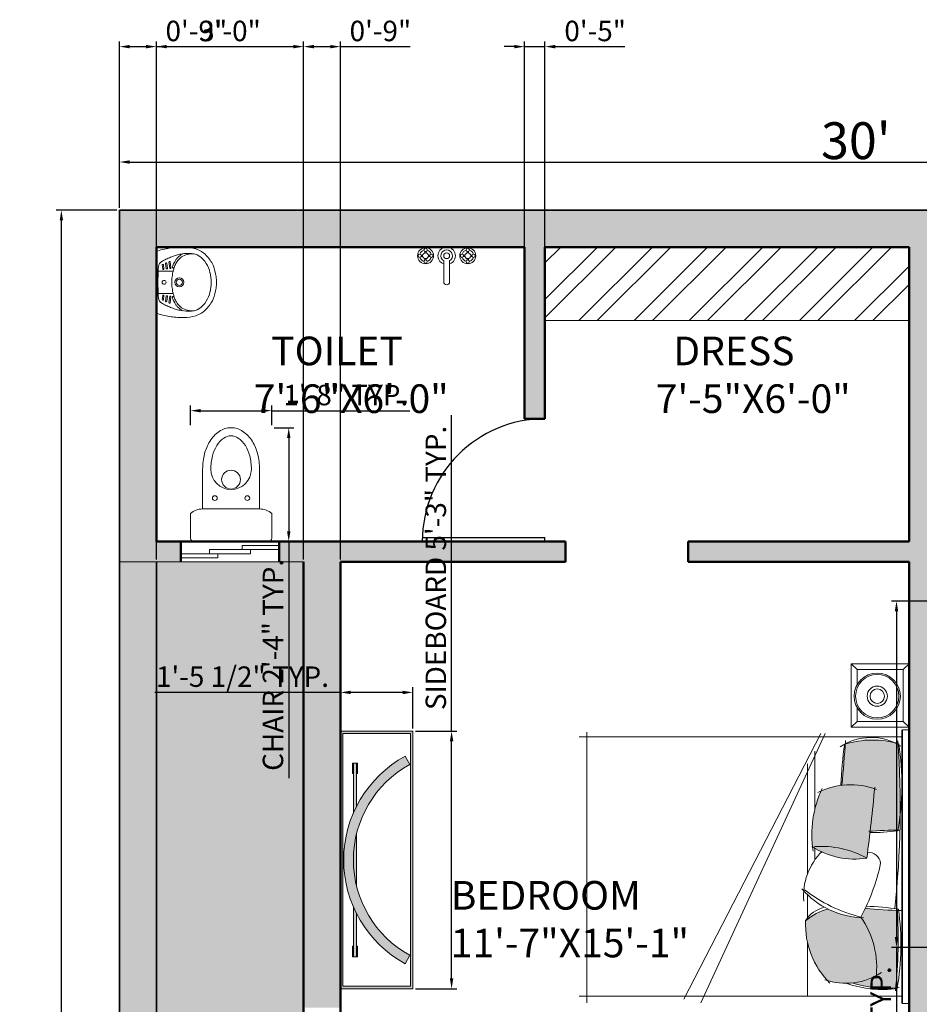
# Model space of a CAD drawing. Units: inches. Extents: x 1734 to 4011, y 1071 to 1891.
# Tile 18 of 27: x 3092 to 3311, y 1638 to 1878. Entities that reach past the tile are written whole.
import ezdxf

# ---------------------------------------------------------------- set-up
doc = ezdxf.new("R2010")
doc.units = ezdxf.units.IN
for name, color, linetype, lineweight in [('0.10', 252, 'Continuous', 9), ('0.15', 34, 'Continuous', 15), ('A-ANNO-DIMS', 2, 'Continuous', 18), ('A-AREA-IDEN', 3, 'Continuous', 18), ('A-DOOR', 3, 'Continuous', 25), ('A-FLOR-FIXT', 9, 'Continuous', 18), ('A-FLOR-PATT', 252, 'Continuous', 13), ('A-FURN', 8, 'Continuous', 18), ('A-FURN-PATT', 252, 'Continuous', 13), ('A-GLAZ', 4, 'Continuous', 18), ('A-WALL', 7, 'Continuous', 50), ('A-WALL-PATT', 8, 'Continuous', 13), ('aparador', 36, 'Continuous', 9), ('C-PROP', 1, 'Continuous', 35), ('moveis', 254, 'Continuous', 5)]:
    doc.layers.add(name, color=color, linetype=linetype, lineweight=lineweight)
doc.styles.get("Standard").update_dxf_attribs({"font": 'arial.ttf'})
doc.dimstyles.new('ISO-25', dxfattribs={"dimtxt": 5, "dimasz": 2.5, "dimexe": 1.25, "dimexo": 0.625, "dimtad": 1, "dimdec": 1, "dimlunit": 3, "dimtxsty": 'Standard', "dimcen": 2.5, "dimclrt": 1, "dimadec": 0, "dimazin": 0, "dimtfac": 1, "dimtdec": 1, "dimtmove": 0, "dimatfit": 3, "dimfxl": 1, "dimarcsym": 0})

# ---------------------------------------------------------------- blocks, each defined once
blk = doc.blocks.new('*D70')
at = {"layer": 'A-ANNO-DIMS', "color": 0, "lineweight": -2, "transparency": 16777216}
for p, q in [((3115.99, 1832.44), (3115.99, 1844.85)), ((3475.99, 1832.44), (3475.99, 1844.85)), ((3118.49, 1843.6), (3473.49, 1843.6))]:
    blk.add_line(p, q, dxfattribs=at)
at = {"layer": 'A-ANNO-DIMS', "color": 0, "transparency": 16777216}
for points in [[(3118.49, 1844.02), (3118.49, 1843.18), (3115.99, 1843.6)], [(3473.49, 1844.02), (3473.49, 1843.18), (3475.99, 1843.6)]]:
    blk.add_solid(points, dxfattribs=at)
at = {"layer": 'Defpoints', "color": 0, "transparency": 16777216}
for p in [(3475.99, 1843.6), (3115.99, 1831.82), (3475.99, 1831.82)]:
    blk.add_point(p, dxfattribs=at)
at = {"layer": 'A-ANNO-DIMS', "color": 0, "transparency": 16777216, "insert": (3295.99, 1848.82), "char_height": 5, "attachment_point": 5}
blk.add_mtext("{\\H1.8x;30'}", dxfattribs=at)
blk = doc.blocks.new('*D66')
at = {"layer": 'A-ANNO-DIMS', "color": 0, "lineweight": -2, "transparency": 16777216}
for p, q in [((3115.37, 1831.82), (3100.52, 1831.82)), ((3101.77, 1114.32), (3101.77, 1829.32)), ((3115.37, 1111.82), (3100.52, 1111.82))]:
    blk.add_line(p, q, dxfattribs=at)
at = {"layer": 'A-ANNO-DIMS', "color": 0, "transparency": 16777216}
for points in [[(3101.36, 1829.32), (3102.19, 1829.32), (3101.77, 1831.82)], [(3101.36, 1114.32), (3102.19, 1114.32), (3101.77, 1111.82)]]:
    blk.add_solid(points, dxfattribs=at)
at = {"layer": 'Defpoints', "color": 0, "transparency": 16777216}
for p in [(3101.77, 1831.82), (3115.99, 1831.82), (3115.99, 1111.82)]:
    blk.add_point(p, dxfattribs=at)
at = {"layer": 'A-ANNO-DIMS', "color": 0, "transparency": 16777216, "insert": (3096.55, 1471.82), "char_height": 5, "attachment_point": 5, "rotation": 90}
blk.add_mtext("{\\H1.8x;60'}", dxfattribs=at)
blk = doc.blocks.new("D2 2'6")
for p, q in [((0, 30), (0, 0)), ((1, 30), (1, 0)), ((0, 0), (1, 0))]:
    blk.add_line(p, q)
blk.add_arc((0, 0), 30, 0, 90)
blk = doc.blocks.new('camita')
at = {"layer": '0.10'}
for p, q in [((-0.85, -0.045), (0.85, -0.045)), ((-0.805, -0.045), (-0.805, -2.0485)), ((0.805, -0.045), (0.805, -2.0485)), ((-0.8271, -0.521), (0.8464, -1.2932)), ((-0.8271, -0.5476), (0.8236, -1.3992)), ((-0.7161, -0.585), (-0.3554, -0.585)), ((-0.1136, -0.585), (-0.0485, -0.585)), ((-0.638, -0.63), (0.0434, -0.63)), ((0.1749, -0.63), (0.3179, -0.63)), ((0.4739, -0.63), (0.805, -0.63)), ((-0.8354, -2), (0.8464, -2))]:
    blk.add_line(p, q, dxfattribs=at)
blk.add_lwpolyline([(-0.85, -0.0405), (0.85, -0.0405), (0.85, 0), (-0.85, 0)], close=True, dxfattribs=at)
for centre, radius, start, end in [((-0.4574, -0.2364), 0.3443, 147.50996, 213.83359), ((-0.3639, -5.8457), 5.7909, 83.80731, 94.12107), ((-0.5104, -1.7232), 1.6781, 80.12554, 98.66187), ((2.3534, -0.0532), 2.5803, 180.10628, 184.38541), ((-1.4396, -0.0609), 1.7117, 352.92911, 0.39592), ((0.4863, -1.6286), 1.5781, 80.16015, 98.05996), ((-0.1997, -0.2266), 0.5864, 163.92635, 197.14087), ((-1.5443, -0.2452), 1.3333, 359.93941, 7.55329), ((1.5815, -0.2893), 1.3353, 170.38021, 178.99138), ((0.4524, -3.0675), 2.9996, 83.90257, 93.67595), ((0.0294, -0.1377), 0.7262, 342.58415, 6.00484), ((0.1326, -0.1696), 0.6307, 339.92303, 8.74334), ((-0.007, -0.258), 0.0828, 100.01798, 179.73597), ((-0.2931, -1.4378), 1.2903, 61.97485, 77.84351), ((0.3203, -0.3944), 0.4043, 341.45245, 33.45121), ((-0.0543, -0.3633), 0.4542, 159.30257, 206.50263), ((-1.3301, -9.6748), 9.4985, 82.27078, 84.93989), ((0.6265, -0.7518), 0.5508, 82.96906, 124.67388), ((0.4585, -0.5454), 0.5842, 151.04555, 184.14969), ((-0.5341, -0.3393), 0.4875, 327.26442, 9.0473), ((-0.1986, -0.2742), 0.5159, 310.73945, 359.05759), ((-0.5673, -0.0868), 0.9057, 321.69527, 346.46261), ((-1.8672, -14.986), 14.6323, 84.65974, 85.75157), ((-0.4598, 1.4861), 1.9092, 260.95299, 268.65169), ((-0.2002, 0.064), 0.6673, 244.78094, 279.06058), ((0.179, -0.272), 0.3828, 224.52836, 275.22287), ((0.4384, -0.4834), 0.1898, 193.68485, 236.70352), ((0.5707, -0.4317), 0.3145, 192.93877, 221.96363), ((0.3612, -0.133), 0.5096, 267.25889, 315.29965)]:
    blk.add_arc(centre, radius, start, end, dxfattribs=at)
blk = doc.blocks.new('VELADOR')
at = {"layer": '0.15'}
for p, q in [((-0.2475, 0), (-0.2025, -0.045)), ((0.2475, 0), (0.2025, -0.045)), ((-0.2025, -0.405), (-0.2475, -0.45)), ((0.2475, -0.45), (0.2025, -0.405))]:
    blk.add_line(p, q, dxfattribs=at)
blk.add_lwpolyline([(-0.2475, 0), (-0.2475, -0.45), (0.2475, -0.45), (0.2475, 0)], close=True, dxfattribs=at)
blk.add_lwpolyline([(0.0921, -0.405), (0.2025, -0.405), (0.2025, -0.045), (-0.2025, -0.045), (-0.2025, -0.405), (-0.0818, -0.405)], dxfattribs=at)
for radius in [0.18, 0.1688, 0.0788, 0.0563]:
    blk.add_circle((0.0052, -0.2474), radius, dxfattribs=at)
blk = doc.blocks.new('Aparador ORGANICA Formatto')
at = {"layer": 'aparador', "ltscale": 0.3}
h = blk.add_hatch(color=256, dxfattribs=at)
h.dxf.hatch_style = 1
h.set_gradient(color1=(118, 213, 123), color2=(52, 168, 57), one_color=1, tint=0.43, name='INVCURVED')
h.paths.add_polyline_path([(0.8, 0.45), (-0.8, 0.45), (-0.8, 0), (0.8, 0)])
h.paths.add_polyline_path([(0.785, 0.435), (0.785, 0.015), (-0.785, 0.015), (-0.785, 0.435)], flags=16)
h.paths.add_polyline_path([(0.2911, 0.3699), (0.5365, 0.3699), (0.5365, 0.3757), (0.6011, 0.3757), (0.6011, 0.3699), (0.6011, 0.3499), (0.6011, 0.3441), (0.5365, 0.3441), (0.5365, 0.3499), (0.3338, 0.3499, -0.150336), (0.6449, 0.0488), (0.5923, 0.0199, 0.208852), (0.1632, 0.3499), (-0.1632, 0.3499, 0.208852), (-0.5923, 0.0199), (-0.6449, 0.0488, -0.150336), (-0.3338, 0.3499), (-0.5365, 0.3499), (-0.5365, 0.3441), (-0.6011, 0.3441), (-0.6011, 0.3499), (-0.6011, 0.3699), (-0.6011, 0.3757), (-0.5365, 0.3757), (-0.5365, 0.3699), (-0.2911, 0.3699, -0.206106)], flags=0)
h = blk.add_hatch(color=256, dxfattribs=at)
h.dxf.hatch_style = 1
h.set_gradient(color1=(135, 92, 69), color2=(0, 0, 0), one_color=1, name='INVCURVED')
h.paths.add_polyline_path([(-0.6449, 0.0488), (-0.5923, 0.0199, -0.590888), (0.5923, 0.0199), (0.6449, 0.0488, 0.590888)])
h = blk.add_hatch(color=256, dxfattribs=at)
h.dxf.hatch_style = 1
h.set_gradient(color1=(178, 189, 189), one_color=1, tint=1, name='CYLINDER')
h.paths.add_polyline_path([(-0.5365, 0.3757), (-0.6011, 0.3757), (-0.6011, 0.3699), (-0.5365, 0.3699)])
h.paths.add_polyline_path([(-0.5365, 0.3499), (-0.6011, 0.3499), (-0.6011, 0.3441), (-0.5365, 0.3441)])
h = blk.add_hatch(color=256, dxfattribs=at)
h.dxf.hatch_style = 1
h.set_gradient(color1=(118, 213, 123), color2=(31, 101, 35), one_color=1, tint=0.26, name='INVCURVED')
h.paths.add_polyline_path([(-0.2911, 0.3699), (-0.6011, 0.3699), (-0.6011, 0.3499), (-0.3338, 0.3499, -0.015999)])
h = blk.add_hatch(color=256, dxfattribs=at)
h.dxf.hatch_style = 1
h.set_gradient(color1=(118, 213, 123), color2=(31, 101, 35), one_color=1, tint=0.26, name='INVCURVED')
h.paths.add_polyline_path([(-0.1632, 0.3499), (0.1632, 0.3499, 0.122516)])
h = blk.add_hatch(color=256, dxfattribs=at)
h.dxf.hatch_style = 1
h.set_gradient(color1=(118, 213, 123), color2=(31, 101, 35), one_color=1, tint=0.26, name='INVCURVED')
h.paths.add_polyline_path([(0.6011, 0.3699), (0.2911, 0.3699, -0.015999), (0.3338, 0.3499), (0.6011, 0.3499)])
h = blk.add_hatch(color=256, dxfattribs=at)
h.dxf.hatch_style = 1
h.set_gradient(color1=(178, 189, 189), one_color=1, tint=1, name='CYLINDER')
h.paths.add_polyline_path([(0.6011, 0.3757), (0.5365, 0.3757), (0.5365, 0.3699), (0.6011, 0.3699)])
h.paths.add_polyline_path([(0.6011, 0.3499), (0.5365, 0.3499), (0.5365, 0.3441), (0.6011, 0.3441)])
for p, q in [((-0.5923, 0.0199), (-0.6449, 0.0488)), ((0.5923, 0.0199), (0.6449, 0.0488))]:
    blk.add_line(p, q, dxfattribs=at)
for points in [[(-0.6011, 0.3699), (-0.6011, 0.3757), (-0.5365, 0.3757), (-0.5365, 0.3699)], [(0.6011, 0.3699), (0.6011, 0.3757), (0.5365, 0.3757), (0.5365, 0.3699)], [(-0.5365, 0.3499), (-0.5365, 0.3441), (-0.6011, 0.3441), (-0.6011, 0.3499)], [(0.5365, 0.3499), (0.5365, 0.3441), (0.6011, 0.3441), (0.6011, 0.3499)]]:
    blk.add_lwpolyline(points, dxfattribs=at)
for radius in [0.7362, 0.6762]:
    blk.add_arc((0, -0.3063), radius, 28.84335, 151.15665, dxfattribs=at)
at = {"layer": 'moveis', "ltscale": 0.3}
for p, q in [((-0.6011, 0.3699), (-0.6011, 0.3499)), ((-0.2911, 0.3699), (-0.6011, 0.3699)), ((0.2911, 0.3699), (0.6011, 0.3699)), ((0.6011, 0.3699), (0.6011, 0.3499)), ((-0.6011, 0.3499), (-0.3338, 0.3499)), ((-0.1632, 0.3499), (0.1632, 0.3499)), ((0.6011, 0.3499), (0.3338, 0.3499))]:
    blk.add_line(p, q, dxfattribs=at)
for points in [[(-0.8, 0), (0.8, 0), (0.8, 0.45), (-0.8, 0.45)], [(-0.785, 0.015), (0.785, 0.015), (0.785, 0.435), (-0.785, 0.435)]]:
    blk.add_lwpolyline(points, close=True, dxfattribs=at)
blk = doc.blocks.new('Faucet - Bathroom top')
for p, q in [((-4.107, 0.125), (-4.375, 0.125)), ((-3.75, 0.4788), (-3.75, 0.75)), ((-3.5, 0.482), (-3.5, 0.75)), ((-3.1461, 0.125), (-2.875, 0.125)), ((3.143, 0.125), (2.875, 0.125)), ((3.5, 0.4788), (3.5, 0.75)), ((3.75, 0.482), (3.75, 0.75)), ((4.1039, 0.125), (4.375, 0.125)), ((-4.1039, -0.125), (-4.375, -0.125)), ((-3.75, -0.4821), (-3.75, -0.75)), ((-3.5, -0.4789), (-3.5, -0.75)), ((-3.143, -0.125), (-2.875, -0.125)), ((-0.5, -0.8639), (-0.5, -4.5)), ((0.5, -4.5), (0.5, -0.8631)), ((3.1461, -0.125), (2.875, -0.125)), ((3.5, -0.4821), (3.5, -0.75)), ((3.75, -0.4789), (3.75, -0.75)), ((4.107, -0.125), (4.375, -0.125))]:
    blk.add_line(p, q)
for centre, radius in [((-3.625, 0), 1.375), ((-4.625, 0), 0.2795), ((-3.625, 0), 0.5), ((-3.625, 1), 0.2795), ((-2.625, 0), 0.2795), ((0, 0), 0.5), ((3.625, 0), 1.375), ((2.625, 0), 0.2795), ((3.625, 0), 0.5), ((3.625, 1), 0.2795), ((4.625, 0), 0.2795), ((-3.625, -1), 0.2795), ((3.625, -1), 0.2795)]:
    blk.add_circle(centre, radius)
for centre, radius, start, end in [((-3.625, 0), 1, 105.2407, 164.2093), ((-3.625, 0), 1, 16.44125, 74.07887), ((0, 0), 1.5, 289.6514, 250.3603), ((0, 0), 1, 300.3431, 239.7554), ((3.625, 0), 1, 106.12, 164.0884), ((3.625, 0), 1, 16.23422, 73.90469), ((-3.625, 0), 1, 196.2342, 253.9047), ((-3.625, 0), 1, 286.12, 344.0884), ((3.625, 0), 1, 196.4413, 254.0789), ((3.625, 0), 1, 285.2407, 344.2093), ((0, -4.5), 0.5, 180, 0)]:
    blk.add_arc(centre, radius, start, end)
blk = doc.blocks.new('lavamanos 2')
at = {"layer": '0.15'}
for p, q in [((0, 0.2335), (0, -0.2335)), ((-0.1127, 0.112), (-0.1067, 0.1581)), ((-0.1037, 0.1109), (-0.0978, 0.157)), ((-0.1304, 0.11), (-0.1315, 0.11)), ((-0.0142, 0.087), (-0.13, 0.086)), ((-0.0857, 0.1085), (-0.0807, 0.1466)), ((-0.0767, 0.1074), (-0.0718, 0.1455)), ((-0.0587, 0.105), (-0.0548, 0.1351)), ((-0.0497, 0.1039), (-0.0458, 0.134)), ((-0.1304, -0.11), (-0.1315, -0.11)), ((-0.0142, -0.087), (-0.13, -0.086)), ((-0.1127, -0.112), (-0.1067, -0.1581)), ((-0.1037, -0.1109), (-0.0978, -0.157)), ((-0.0857, -0.1085), (-0.0807, -0.1466)), ((-0.0767, -0.1074), (-0.0718, -0.1455)), ((-0.0587, -0.105), (-0.0548, -0.1351)), ((-0.0497, -0.1039), (-0.0458, -0.134))]:
    blk.add_line(p, q, dxfattribs=at)
for centre, radius in [((-0.178, 0), 0.035), ((-0.178, 0), 0.0235), ((-0.06, 0), 0.015)]:
    blk.add_circle(centre, radius, dxfattribs=at)
for centre, radius, start, end in [((-0.2419, 0.0663), 0.2023, 108.1945, 135.36859), ((-0.2035, -0.0862), 0.3593, 91.20299, 106.42552), ((-0.2208, -0.6855), 0.9585, 86.55138, 89.41308), ((-0.2121, -0.5476), 0.8204, 83.12241, 86.5796), ((5.8279, 30.215), 30.5319, 258.77821, 258.87599), ((-0.1265, -0.0657), 0.3287, 69.06009, 78.82181), ((-0.0202, 0.212), 0.0314, 54.79491, 69.06009), ((-0.005, 0.2335), 0.005, 0, 54.79491), ((-0.1663, 0.0005), 0.3024, 136.57187, 154.32772), ((-0.2422, 0.0655), 0.1638, 121.99295, 150.58892), ((-0.2657, 0.1037), 0.119, 92.47742, 122.14108), ((-0.2765, 0.0677), 0.1528, 57.2491, 95.54005), ((-0.2442, -0.0128), 0.2368, 77.24819, 96.46321), ((-0.2765, 0.0677), 0.1678, 56.87663, 64.99714), ((-0.3662, -0.002), 0.2627, 40.35252, 49.00458), ((-0.2222, 0.0026), 0.2177, 71.98488, 82.01242), ((-0.3662, -0.002), 0.2777, 40.35252, 49.22548), ((-0.2374, 0.11), 0.0921, 27.31862, 39.11562), ((-0.3103, -0.315), 0.5472, 69.51913, 73.49118), ((-0.2374, 0.11), 0.1071, 27.57433, 39.11562), ((-0.3494, 0.0363), 0.2408, 22.19214, 30.78376), ((-0.2991, -0.2855), 0.5156, 65.23004, 69.53785), ((-0.1022, 0.1575), 0.0045, 352.61396, 172.61396), ((-0.2784, -0.2408), 0.4663, 60.24131, 65.2382), ((-0.0648, 0.1184), 0.049, 1.58272, 68.62081), ((-0.0557, -0.0178), 0.4111, 158.70106, 171.31016), ((-0.1999, 0.0263), 0.2202, 147.11565, 167.44248), ((-0.3494, 0.0363), 0.2258, 22.33605, 30.8927), ((-1.2664, -0.2389), 1.1824, 16.36313, 17.77674), ((-0.1315, 0.117), 0.007, 197.40991, 270.49494), ((0.1853, 0.1648), 0.325, 192.53887, 196.70718), ((-0.1305, 0.117), 0.007, 270.49494, 17.39527), ((-1.2664, -0.2389), 1.1974, 17.39527, 17.80495), ((-0.1082, 0.1115), 0.0045, 172.61396, 352.61396), ((-0.0812, 0.108), 0.0045, 172.61396, 352.61396), ((-0.0763, 0.146), 0.0045, 352.61396, 172.61396), ((-0.0542, 0.1045), 0.0045, 172.61396, 352.61396), ((-0.0503, 0.1345), 0.0045, 352.61396, 172.61396), ((-2.1477, 0.0009), 2.1352, 359.97535, 3.19009), ((-0.2093, 0.0056), 0.2558, 171.31016, 181.26266), ((-0.2093, -0.0056), 0.2558, 178.73734, 188.68984), ((0.4664, -0.0834), 0.8953, 169.86317, 174.65802), ((0.4664, 0.0834), 0.8953, 185.34198, 190.13683), ((0.3887, 0.121), 0.517, 185.50529, 189.81306), ((-0.7181, -0.0071), 0.5987, 0.67647, 3.82165), ((-0.7181, 0.0071), 0.5987, 356.17835, 359.32353), ((-2.1477, -0.0009), 2.1352, 356.80991, 0.02465), ((-0.0557, 0.0178), 0.4111, 188.68984, 201.29894), ((-0.1999, -0.0263), 0.2202, 192.55752, 212.88435), ((0.1853, -0.1648), 0.325, 163.29282, 167.46113), ((0.3887, -0.1209), 0.517, 170.18694, 174.49471), ((-0.1663, -0.0005), 0.3024, 205.67228, 223.42813), ((-0.2422, -0.0655), 0.1638, 209.41108, 238.00705), ((-0.2374, -0.1099), 0.0921, 320.88438, 332.68138), ((-0.3494, -0.0363), 0.2258, 329.1073, 337.66395), ((-0.3494, -0.0363), 0.2408, 329.21624, 337.80786), ((-1.2664, 0.2389), 1.1824, 342.22326, 343.63687), ((-0.1315, -0.117), 0.007, 89.50506, 162.59009), ((-0.1305, -0.117), 0.007, 342.60473, 89.50506), ((-1.2664, 0.2389), 1.1974, 342.19505, 342.60473), ((-0.1082, -0.1115), 0.0045, 7.38604, 187.38604), ((-0.0812, -0.108), 0.0045, 7.38604, 187.38604), ((-0.0763, -0.146), 0.0045, 187.38604, 7.38604), ((-0.0542, -0.1045), 0.0045, 7.38604, 187.38604), ((-0.0503, -0.1345), 0.0045, 187.38604, 7.38604), ((-0.0648, -0.1184), 0.049, 291.37919, 358.41728), ((-0.2419, -0.0663), 0.2023, 224.63141, 251.8055), ((-0.2657, -0.1036), 0.119, 237.85892, 267.52258), ((-0.2765, -0.0677), 0.1528, 264.45995, 302.7509), ((-0.2442, 0.0128), 0.2368, 263.53679, 282.75181), ((-0.2765, -0.0677), 0.1678, 295.00286, 303.12337), ((-0.3662, 0.002), 0.2627, 310.99542, 319.64748), ((-0.2222, -0.0026), 0.2177, 277.98758, 288.01512), ((-0.3662, 0.002), 0.2777, 310.77452, 319.64748), ((-0.3103, 0.315), 0.5472, 286.50882, 290.48087), ((-0.2374, -0.1099), 0.1071, 320.88438, 332.42567), ((-0.2991, 0.2855), 0.5156, 290.46215, 294.76996), ((-0.1022, -0.1575), 0.0045, 187.38604, 7.38604), ((-0.2784, 0.2408), 0.4663, 294.7618, 299.75869), ((-0.2035, 0.0862), 0.3593, 253.57448, 268.79701), ((-0.2208, 0.6855), 0.9585, 270.58692, 273.44862), ((-0.2121, 0.5476), 0.8204, 273.4204, 276.87759), ((5.8279, -30.215), 30.5319, 101.12401, 101.22179), ((-0.1265, 0.0657), 0.3287, 281.17819, 290.93991), ((-0.0202, -0.212), 0.0314, 290.93991, 305.20509), ((-0.005, -0.2335), 0.005, 305.20509, 0)]:
    blk.add_arc(centre, radius, start, end, dxfattribs=at)
blk = doc.blocks.new('rreerr')
blk.add_lwpolyline([(2512.8529, 833.5601, 0.205217), (2512.9279, 833.5883), (2512.9279, 833.7401, 0.414214), (2512.9079, 833.7601), (2512.4479, 833.7601, 0.414214), (2512.4279, 833.7401), (2512.4279, 833.5883, 0.205217), (2512.5029, 833.5601)], format="xyb")
for points in [[(2512.5468, 833.1438, 0.107027), (2512.6056, 833.0819, 0.150548), (2512.6779, 833.0596, 0.150548), (2512.7502, 833.0819, 0.107027), (2512.809, 833.1438, 0.075071), (2512.8412, 833.2206, 0.0618), (2512.8529, 833.3151), (2512.8529, 833.5601), (2512.5029, 833.5601), (2512.5029, 833.3151, 0.0618), (2512.5146, 833.2206, 0.075071)], [(2512.5631, 833.2328, 0.075071), (2512.5895, 833.1698, 0.107027), (2512.6338, 833.1232, 0.150548), (2512.6779, 833.1096, 0.150548), (2512.722, 833.1232, 0.107027), (2512.7663, 833.1698, 0.075071), (2512.7927, 833.2328, 0.0618), (2512.8029, 833.3151, 1), (2512.5529, 833.3151, 0.0618)]]:
    blk.add_lwpolyline(points, format="xyb", close=True)
for centre, radius in [((2512.5779, 833.493), 0.0146), ((2512.7779, 833.493), 0.0146), ((2512.6775, 833.3793), 0.0579)]:
    blk.add_circle(centre, radius)
blk = doc.blocks.new('*D83')
at = {"layer": 'A-ANNO-DIMS', "color": 0, "lineweight": -2, "transparency": 16777216}
for p, q in [((3197.16, 1704.46), (3197.16, 1781.74)), ((3188.34, 1704.46), (3198.41, 1704.46)), ((3197.16, 1643.97), (3197.16, 1701.96)), ((3188.34, 1641.47), (3198.41, 1641.47))]:
    blk.add_line(p, q, dxfattribs=at)
at = {"layer": 'A-ANNO-DIMS', "color": 0, "transparency": 16777216}
for points in [[(3196.74, 1701.96), (3197.58, 1701.96), (3197.16, 1704.46)], [(3196.74, 1643.97), (3197.58, 1643.97), (3197.16, 1641.47)]]:
    blk.add_solid(points, dxfattribs=at)
at = {"layer": 'Defpoints', "color": 0, "transparency": 16777216}
for p in [(3187.71, 1704.46), (3197.16, 1704.46), (3187.71, 1641.47)]:
    blk.add_point(p, dxfattribs=at)
at = {"layer": 'A-ANNO-DIMS', "color": 1, "transparency": 16777216, "insert": (3193.95, 1744.35), "char_height": 5, "attachment_point": 5, "rotation": 90}
blk.add_mtext('SIDEBOARD 5\'-3" TYP.', dxfattribs=at)
blk = doc.blocks.new('*D84')
at = {"layer": 'A-ANNO-DIMS', "color": 0, "lineweight": -2, "transparency": 16777216}
for p, q in [((3169.99, 1705.08), (3169.99, 1715.16)), ((3187.71, 1705.08), (3187.71, 1715.16)), ((3169.99, 1713.91), (3124.59, 1713.91)), ((3185.21, 1713.91), (3172.49, 1713.91))]:
    blk.add_line(p, q, dxfattribs=at)
at = {"layer": 'A-ANNO-DIMS', "color": 0, "transparency": 16777216}
for points in [[(3172.49, 1714.32), (3172.49, 1713.49), (3169.99, 1713.91)], [(3185.21, 1714.32), (3185.21, 1713.49), (3187.71, 1713.91)]]:
    blk.add_solid(points, dxfattribs=at)
at = {"layer": 'Defpoints', "color": 0, "transparency": 16777216}
for p in [(3169.99, 1713.91), (3169.99, 1704.46), (3187.71, 1704.46)]:
    blk.add_point(p, dxfattribs=at)
at = {"layer": 'A-ANNO-DIMS', "color": 1, "transparency": 16777216, "insert": (3146.04, 1717.12), "char_height": 5, "attachment_point": 5}
blk.add_mtext('1\'-5 1/2" TYP.', dxfattribs=at)
blk = doc.blocks.new('*D93')
at = {"layer": 'A-ANNO-DIMS', "color": 0, "lineweight": -2, "transparency": 16777216}
for p, q in [((3153.81, 1778.63), (3158.6, 1778.63)), ((3157.35, 1776.13), (3157.35, 1753.32)), ((3153.81, 1750.82), (3158.6, 1750.82)), ((3157.35, 1750.82), (3157.35, 1692.98))]:
    blk.add_line(p, q, dxfattribs=at)
at = {"layer": 'A-ANNO-DIMS', "color": 0, "transparency": 16777216}
for points in [[(3156.94, 1776.13), (3157.77, 1776.13), (3157.35, 1778.63)], [(3156.94, 1753.32), (3157.77, 1753.32), (3157.35, 1750.82)]]:
    blk.add_solid(points, dxfattribs=at)
at = {"layer": 'Defpoints', "color": 0, "transparency": 16777216}
for p in [(3153.18, 1778.63), (3153.18, 1750.82), (3157.35, 1750.82)]:
    blk.add_point(p, dxfattribs=at)
at = {"layer": 'A-ANNO-DIMS', "color": 1, "transparency": 16777216, "insert": (3154.14, 1720.65), "char_height": 5, "attachment_point": 5, "rotation": 90}
blk.add_mtext('CHAIR 2\'-4" TYP.', dxfattribs=at)
blk = doc.blocks.new('*D94')
at = {"layer": 'A-ANNO-DIMS', "color": 0, "lineweight": -2, "transparency": 16777216}
for p, q in [((3133.33, 1779.25), (3133.33, 1784.05)), ((3153.18, 1779.25), (3153.18, 1784.05)), ((3135.83, 1782.8), (3150.68, 1782.8)), ((3153.18, 1782.8), (3186.94, 1782.8))]:
    blk.add_line(p, q, dxfattribs=at)
at = {"layer": 'A-ANNO-DIMS', "color": 0, "transparency": 16777216}
for points in [[(3135.83, 1783.22), (3135.83, 1782.38), (3133.33, 1782.8)], [(3150.68, 1783.22), (3150.68, 1782.38), (3153.18, 1782.8)]]:
    blk.add_solid(points, dxfattribs=at)
at = {"layer": 'Defpoints', "color": 0, "transparency": 16777216}
for p in [(3153.18, 1782.8), (3133.33, 1778.63), (3153.18, 1778.63)]:
    blk.add_point(p, dxfattribs=at)
at = {"layer": 'A-ANNO-DIMS', "color": 1, "transparency": 16777216, "insert": (3171.31, 1785.98), "char_height": 5, "attachment_point": 5}
blk.add_mtext('1\'-8" TYP.', dxfattribs=at)
blk = doc.blocks.new('*D99')
at = {"layer": 'A-ANNO-DIMS', "color": 0, "lineweight": -2, "transparency": 16777216}
for p, q in [((3317.99, 1736.23), (3304.67, 1736.23)), ((3305.92, 1733.73), (3305.92, 1654.07)), ((3317.99, 1651.57), (3304.67, 1651.57)), ((3305.92, 1651.57), (3305.92, 1564.03))]:
    blk.add_line(p, q, dxfattribs=at)
at = {"layer": 'A-ANNO-DIMS', "color": 0, "transparency": 16777216}
for points in [[(3305.5, 1733.73), (3306.34, 1733.73), (3305.92, 1736.23)], [(3305.5, 1654.07), (3306.34, 1654.07), (3305.92, 1651.57)]]:
    blk.add_solid(points, dxfattribs=at)
at = {"layer": 'Defpoints', "color": 0, "transparency": 16777216}
for p in [(3318.62, 1736.23), (3305.92, 1651.57), (3318.62, 1651.57)]:
    blk.add_point(p, dxfattribs=at)
at = {"layer": 'A-ANNO-DIMS', "color": 1, "transparency": 16777216, "insert": (3302.71, 1606.55), "char_height": 5, "attachment_point": 5, "rotation": 90}
blk.add_mtext('DINING SET 7\'-0 1/2" TYP.', dxfattribs=at)
blk = doc.blocks.new('*D119')
at = {"layer": 'A-ANNO-DIMS', "color": 0, "lineweight": -2, "transparency": 16777216}
for p, q in [((3115.99, 1832.44), (3115.99, 1873.07)), ((3118.49, 1871.82), (3122.49, 1871.82)), ((3124.99, 1823.44), (3124.99, 1873.07)), ((3124.99, 1871.82), (3142.03, 1871.82))]:
    blk.add_line(p, q, dxfattribs=at)
at = {"layer": 'A-ANNO-DIMS', "color": 0, "transparency": 16777216}
for points in [[(3118.49, 1872.24), (3118.49, 1871.4), (3115.99, 1871.82)], [(3122.49, 1872.24), (3122.49, 1871.4), (3124.99, 1871.82)]]:
    blk.add_solid(points, dxfattribs=at)
at = {"layer": 'Defpoints', "color": 0, "transparency": 16777216}
for p in [(3124.99, 1871.82), (3115.99, 1831.82), (3124.99, 1822.82)]:
    blk.add_point(p, dxfattribs=at)
at = {"layer": 'A-ANNO-DIMS', "color": 1, "transparency": 16777216, "insert": (3134.76, 1875), "char_height": 5, "attachment_point": 5}
blk.add_mtext('0\'-9"', dxfattribs=at)
blk = doc.blocks.new('*D121')
at = {"layer": 'A-ANNO-DIMS', "color": 0, "lineweight": -2, "transparency": 16777216}
for p, q in [((3212.49, 1871.82), (3209.99, 1871.82)), ((3214.99, 1781.44), (3214.99, 1873.07)), ((3214.99, 1871.82), (3219.99, 1871.82)), ((3219.99, 1781.44), (3219.99, 1873.07)), ((3222.49, 1871.82), (3239.53, 1871.82))]:
    blk.add_line(p, q, dxfattribs=at)
at = {"layer": 'A-ANNO-DIMS', "color": 0, "transparency": 16777216}
for points in [[(3212.49, 1872.24), (3212.49, 1871.4), (3214.99, 1871.82)], [(3222.49, 1872.24), (3222.49, 1871.4), (3219.99, 1871.82)]]:
    blk.add_solid(points, dxfattribs=at)
at = {"layer": 'Defpoints', "color": 0, "transparency": 16777216}
for p in [(3219.99, 1871.82), (3214.99, 1780.82), (3219.99, 1780.82)]:
    blk.add_point(p, dxfattribs=at)
at = {"layer": 'A-ANNO-DIMS', "color": 1, "transparency": 16777216, "insert": (3232.26, 1875), "char_height": 5, "attachment_point": 5}
blk.add_mtext('0\'-5"', dxfattribs=at)
blk = doc.blocks.new('*D122')
at = {"layer": 'A-ANNO-DIMS', "color": 0, "lineweight": -2, "transparency": 16777216}
for p, q in [((3124.99, 1746.44), (3124.99, 1873.07)), ((3127.49, 1871.82), (3158.49, 1871.82)), ((3160.99, 1746.44), (3160.99, 1873.07))]:
    blk.add_line(p, q, dxfattribs=at)
at = {"layer": 'A-ANNO-DIMS', "color": 0, "transparency": 16777216}
for points in [[(3127.49, 1872.24), (3127.49, 1871.4), (3124.99, 1871.82)], [(3158.49, 1872.24), (3158.49, 1871.4), (3160.99, 1871.82)]]:
    blk.add_solid(points, dxfattribs=at)
at = {"layer": 'Defpoints', "color": 0, "transparency": 16777216}
for p in [(3160.99, 1871.82), (3124.99, 1745.82), (3160.99, 1745.82)]:
    blk.add_point(p, dxfattribs=at)
at = {"layer": 'A-ANNO-DIMS', "color": 1, "transparency": 16777216, "insert": (3142.99, 1875), "char_height": 5, "attachment_point": 5}
blk.add_mtext('3\'-0"', dxfattribs=at)
blk = doc.blocks.new('*D123')
at = {"layer": 'A-ANNO-DIMS', "color": 0, "lineweight": -2, "transparency": 16777216}
for p, q in [((3160.99, 1746.44), (3160.99, 1873.07)), ((3163.49, 1871.82), (3167.49, 1871.82)), ((3169.99, 1746.44), (3169.99, 1873.07)), ((3169.99, 1871.82), (3187.03, 1871.82))]:
    blk.add_line(p, q, dxfattribs=at)
at = {"layer": 'A-ANNO-DIMS', "color": 0, "transparency": 16777216}
for points in [[(3163.49, 1872.24), (3163.49, 1871.4), (3160.99, 1871.82)], [(3167.49, 1872.24), (3167.49, 1871.4), (3169.99, 1871.82)]]:
    blk.add_solid(points, dxfattribs=at)
at = {"layer": 'Defpoints', "color": 0, "transparency": 16777216}
for p in [(3169.99, 1871.82), (3160.99, 1745.82), (3169.99, 1745.82)]:
    blk.add_point(p, dxfattribs=at)
at = {"layer": 'A-ANNO-DIMS', "color": 1, "transparency": 16777216, "insert": (3179.76, 1875), "char_height": 5, "attachment_point": 5}
blk.add_mtext('0\'-9"', dxfattribs=at)

msp = doc.modelspace()

# ---------------------------------------------------------------- hatches: boundary and pattern name
at = {"layer": 'A-FLOR-PATT'}
h = msp.add_hatch(color=256, dxfattribs=at)
h.dxf.hatch_style = 1
h.paths.add_polyline_path([(3124.99, 1745.82), (3115.99, 1745.82), (3115.99, 1111.82), (3171.99, 1111.82), (3171.99, 1120.82), (3124.99, 1120.82)])
h = msp.add_hatch(color=256, dxfattribs=at)
h.dxf.hatch_style = 1
h.paths.add_polyline_path([(3160.99, 1745.82), (3124.99, 1745.82), (3124.99, 1312.82), (3160.99, 1312.82), (3160.99, 1529.82)])
at = {"layer": 'A-FURN-PATT'}
h = msp.add_hatch(dxfattribs=at)
h.set_pattern_fill('ANSI32', color=256)
h.set_pattern_definition([(45, (1357.344, -12.241), (-6.735192, 6.735192), []), (45, (1361.834, -12.241), (-6.735192, 6.735192), [])])
h.paths.add_polyline_path([(3308.99, 1822.82), (3219.99, 1822.82), (3219.99, 1804.82), (3308.99, 1804.82)])
h.paths.add_polyline_path([(3253.99, 1453.82), (3169.99, 1453.82), (3169.99, 1435.82), (3253.99, 1435.82)])
h.paths.add_polyline_path([(3183.49, 1440.04), (3232.95, 1440.04), (3232.95, 1450.34), (3183.49, 1450.34)], flags=24)
h = msp.add_hatch(color=256, dxfattribs=at)
h.dxf.hatch_style = 1
h.paths.add_polyline_path([(3306.31, 1701.16, 0.020657), (3305.31, 1701.67, 0.131047), (3293.42, 1701.29, -0.004387), (3292.57, 1691.22, -0.113891), (3300.56, 1690.35, -0.006967), (3299.49, 1679.98, -0.016701), (3306.27, 1680.25, 0.015442), (3306.83, 1684.29, 0.01851)])
h.paths.add_polyline_path([(3306.11, 1660.61, -0.029051), (3298.3, 1661.12, -0.011742), (3297.23, 1658.99, -0.175864), (3300.99, 1644.68, -0.098488), (3295.05, 1642.86, 0.094792), (3305.72, 1641.65, 0.040212)])
h = msp.add_hatch(color=256, dxfattribs=at)
h.dxf.hatch_style = 1
h.paths.add_polyline_path([(3300.56, 1690.35, 0.189536), (3287.48, 1689.83, 0.134508), (3285.42, 1676.1, 0.181694), (3298.65, 1673.39, 0.011408)])
h.paths.add_polyline_path([(3297.32, 1658.85, -0.104045), (3289.22, 1660.92, 0.127326), (3283.71, 1658.06, 0.202559), (3289.1, 1643.4, 0.194952), (3300.99, 1644.68, 0.173835)])
at = {"layer": 'A-WALL-PATT'}
h = msp.add_hatch(color=256, dxfattribs=at)
h.dxf.hatch_style = 1
h.paths.add_polyline_path([(3475.99, 1831.82), (3115.99, 1831.82), (3115.99, 1745.82), (3130.99, 1745.82), (3130.99, 1750.82), (3124.99, 1750.82), (3124.99, 1822.82), (3214.99, 1822.82), (3214.99, 1780.82), (3219.99, 1780.82), (3219.99, 1822.82), (3308.99, 1822.82), (3308.99, 1750.82), (3254.99, 1750.82), (3254.99, 1745.82), (3308.99, 1745.82), (3308.99, 1604.82), (3313.99, 1604.82), (3313.99, 1745.82), (3366.99, 1745.82), (3366.99, 1750.82), (3313.99, 1750.82), (3313.99, 1822.82), (3401.99, 1822.82), (3401.99, 1750.82), (3396.99, 1750.82), (3396.99, 1745.82), (3411.99, 1745.82), (3411.99, 1750.82), (3406.99, 1750.82), (3406.99, 1822.82), (3466.99, 1822.82), (3466.99, 1750.82), (3441.99, 1750.82), (3441.99, 1745.82), (3466.99, 1745.82), (3466.99, 1517.82), (3452.49, 1517.82), (3452.49, 1512.82), (3466.99, 1512.82), (3466.99, 1458.82), (3446.49, 1458.82), (3446.49, 1453.82), (3466.99, 1453.82), (3466.99, 1237.82), (3372.99, 1237.82), (3372.99, 1228.82), (3466.99, 1228.82), (3466.99, 1120.82), (3309.99, 1120.82), (3309.99, 1184.82), (3310.99, 1184.82), (3310.99, 1189.82), (3303.99, 1189.82), (3303.99, 1120.82), (3291.99, 1120.82), (3291.99, 1111.82), (3475.99, 1111.82)])
h.paths.add_polyline_path([(3169.99, 1745.82), (3224.99, 1745.82), (3224.99, 1750.82), (3154.99, 1750.82), (3154.99, 1745.82), (3160.99, 1745.82), (3160.99, 1636.82), (3169.99, 1636.82)], flags=17)
h.paths.add_polyline_path([(3169.99, 1588.82), (3160.99, 1588.82), (3160.99, 1559.82), (3313.99, 1559.82), (3313.99, 1568.82), (3308.99, 1568.82), (3308.99, 1564.82), (3169.99, 1564.82)], flags=17)
h.paths.add_polyline_path([(3416.49, 1517.82), (3401.99, 1517.82), (3401.99, 1512.82), (3416.49, 1512.82)], flags=17)
h.paths.add_polyline_path([(3371.99, 1517.82), (3366.99, 1517.82), (3366.99, 1453.82), (3392.49, 1453.82), (3392.49, 1458.82), (3371.99, 1458.82)], flags=17)
h.paths.add_polyline_path([(3258.99, 1529.82), (3160.99, 1529.82), (3160.99, 1494.82), (3169.99, 1494.82), (3169.99, 1524.82), (3253.99, 1524.82), (3253.99, 1520.82), (3258.99, 1520.82)], flags=17)
h.paths.add_polyline_path([(3263.99, 1458.82), (3258.99, 1458.82), (3258.99, 1490.82), (3253.99, 1490.82), (3253.99, 1458.82), (3169.99, 1458.82), (3169.99, 1470.82), (3160.99, 1470.82), (3160.99, 1387.82), (3169.99, 1387.82), (3169.99, 1453.82), (3263.99, 1453.82)], flags=17)
h.paths.add_polyline_path([(3313.99, 1453.82), (3318.99, 1453.82), (3318.99, 1458.82), (3299.99, 1458.82), (3299.99, 1453.82), (3308.99, 1453.82), (3308.99, 1321.82), (3266.49, 1321.82), (3266.49, 1312.82), (3313.99, 1312.82)], flags=17)
h.paths.add_polyline_path([(3212.49, 1321.82), (3169.99, 1321.82), (3169.99, 1339.82), (3160.99, 1339.82), (3160.99, 1312.82), (3212.49, 1312.82)], flags=17)
h.paths.add_polyline_path([(3313.99, 1288.82), (3304.99, 1288.82), (3304.99, 1285.82), (3313.99, 1285.82)], flags=17)
h.paths.add_polyline_path([(3324.99, 1237.82), (3304.99, 1237.82), (3304.99, 1228.82), (3324.99, 1228.82)], flags=17)

# ---------------------------------------------------------------- linework, layer by layer
at = {"layer": 'A-FURN'}
for p, q in [((3219.99, 1804.82), (3308.99, 1804.82)), ((3115.99, 1745.82), (3160.99, 1745.82))]:
    msp.add_line(p, q, dxfattribs=at)
at = {"layer": 'A-GLAZ'}
for p, q in [((3137.99, 1748.82), (3137.99, 1747.82)), ((3154.99, 1748.82), (3137.99, 1748.82)), ((3145.99, 1749.82), (3145.99, 1748.82)), ((3154.99, 1749.82), (3145.99, 1749.82)), ((3147.99, 1748.82), (3147.99, 1747.82)), ((3147.99, 1747.82), (3130.99, 1747.82)), ((3139.99, 1746.82), (3130.99, 1746.82)), ((3139.99, 1747.82), (3139.99, 1746.82))]:
    msp.add_line(p, q, dxfattribs=at)
at = {"layer": 'A-WALL'}
for p, q in [((3124.99, 1822.82), (3214.99, 1822.82)), ((3124.99, 1750.82), (3124.99, 1822.82)), ((3214.99, 1780.82), (3214.99, 1822.82)), ((3219.99, 1822.82), (3308.99, 1822.82)), ((3219.99, 1780.82), (3219.99, 1822.82)), ((3308.99, 1750.82), (3308.99, 1822.82)), ((3214.99, 1780.82), (3219.99, 1780.82)), ((3124.99, 1750.82), (3224.99, 1750.82)), ((3130.99, 1750.82), (3130.99, 1745.82)), ((3154.99, 1750.82), (3154.99, 1745.82)), ((3224.99, 1745.82), (3224.99, 1750.82)), ((3254.99, 1745.82), (3254.99, 1750.82)), ((3254.99, 1750.82), (3308.99, 1750.82)), ((3160.99, 1529.82), (3160.99, 1745.82)), ((3169.99, 1745.82), (3224.99, 1745.82)), ((3169.99, 1564.82), (3169.99, 1745.82)), ((3254.99, 1745.82), (3308.99, 1745.82)), ((3308.99, 1604.82), (3308.99, 1745.82))]:
    msp.add_line(p, q, dxfattribs=at)
at = {"layer": 'C-PROP'}
msp.add_line((3124.99, 1120.82), (3124.99, 1745.82), dxfattribs=at)
msp.add_lwpolyline([(3171.99, 1111.82), (3115.99, 1111.82), (3115.99, 1831.82), (3475.99, 1831.82), (3475.99, 1111.82), (3291.99, 1111.82)], dxfattribs=at)

# ---------------------------------------------------------------- block references
at = {"layer": 'A-DOOR', "rotation": 90.00000000000003}
msp.add_blockref("D2 2'6", (3219.99, 1750.82), dxfattribs=at)
at = {"layer": 'A-FLOR-FIXT'}
for name, p, xscale, yscale, zscale, rotation in [('lavamanos 2', (3124.99, 1814.19), 31.61240364394164, 31.61240364394164, 31.61240364394164, 179.99990349049), ('rreerr', (-96612.57, 34851.93), -39.701, 39.701, 39.701, 180)]:
    msp.add_blockref(name, p, dxfattribs=dict(at, xscale=xscale, yscale=yscale, zscale=zscale, rotation=rotation))
at = {"layer": 'A-FLOR-FIXT', "xscale": 1.424049708253414, "yscale": 1.424049708253414, "zscale": 1.424049708253414}
msp.add_blockref('Faucet - Bathroom top', (3195.96, 1820.69), dxfattribs=at)
at = {"layer": 'A-FURN'}
for name, p, xscale, yscale, zscale, rotation in [('VELADOR', (3308.99, 1713.15), 31.41542173157097, 31.41542173157097, 31.41542173157097, 270), ('camita', (3308.99, 1671.32), 39.375, 39.375, 39.375, 270), ('Aparador ORGANICA Formatto', (3187.71, 1672.96), 39.3701, 39.3701, 39.3701, 90)]:
    msp.add_blockref(name, p, dxfattribs=dict(at, xscale=xscale, yscale=yscale, zscale=zscale, rotation=rotation))

# ---------------------------------------------------------------- texts
at = {"layer": 'A-AREA-IDEN', "char_height": 7, "attachment_point": 1}
for s, heights, insert in [('  TOILET\\P7\'-6"X6\'-0"', [18.94], (3148.8, 1800.91)), ('  DRESS\\P7\'-5"X6\'-0"', [18.94], (3247.07, 1800.91)), ('BEDROOM\\P11\'-7"X15\'-1"', [0], (3196.95, 1667.8))]:
    msp.add_mtext_dynamic_manual_height_columns(s, width=86.9528, gutter_width=12.5, heights=heights, dxfattribs=dict(at, insert=insert))

# ---------------------------------------------------------------- dimensions: what is measured, and where the dimension line sits
at = {"layer": 'A-ANNO-DIMS'}
for base, p1, p2, picture, middle in [((3124.99, 1871.82), (3115.99, 1831.82), (3124.99, 1822.82), '*D119', (3134.76, 1875)), ((3160.99, 1871.82), (3124.99, 1745.82), (3160.99, 1745.82), '*D122', (3142.99, 1875)), ((3169.99, 1871.82), (3160.99, 1745.82), (3169.99, 1745.82), '*D123', (3179.76, 1875)), ((3219.99, 1871.82), (3214.99, 1780.82), (3219.99, 1780.82), '*D121', (3232.26, 1875))]:
    dim = msp.add_linear_dim(base=base, p1=p1, p2=p2, dimstyle='ISO-25', override={"dimdec": 1, "dimlfac": 1, "dimrnd": 0, "dimzin": 1, "dimdsep": 46, "dimlunit": 4, "dimfrac": 2}, dxfattribs=at)
    dim.commit()
    dim.dimension.update_dxf_attribs({"geometry": picture, "text_midpoint": middle})
for base, p1, p2, text, override, picture, middle in [((3475.99, 1843.6), (3115.99, 1831.82), (3475.99, 1831.82), '{\\H1.8x;<>}', {"dimclrd": 0, "dimclre": 0, "dimclrt": 0}, '*D70', (3295.99, 1848.82)), ((3153.1827, 1782.7987), (3133.3322, 1778.6275), (3153.1827, 1778.6275), '<> TYP.', {"dimdec": 1, "dimrnd": 0, "dimzin": 1, "dimlunit": 4, "dimfrac": 2}, '*D94', (3171.3111, 1785.9766))]:
    dim = msp.add_linear_dim(base=base, p1=p1, p2=p2, text=text, dimstyle='ISO-25', override=override, dxfattribs=at)
    dim.commit()
    dim.dimension.update_dxf_attribs({"geometry": picture, "text_midpoint": middle})
for base, p1, p2, angle, text, override, picture, middle in [((3101.77, 1831.82), (3115.99, 1111.82), (3115.99, 1831.82), 90, '{\\H1.8x;<>}', {"dimclrd": 0, "dimclre": 0, "dimclrt": 0}, '*D66', (3096.55, 1471.82)), ((3197.16, 1704.46), (3187.71, 1641.47), (3187.71, 1704.46), 90, 'SIDEBOARD <> TYP.', {"dimdec": 1, "dimrnd": 0, "dimzin": 1, "dimlunit": 4, "dimfrac": 2}, '*D83', (3193.95, 1744.35)), ((3157.35, 1750.82), (3153.18, 1778.63), (3153.18, 1750.82), 270, 'CHAIR <> TYP.', {"dimdec": 1, "dimrnd": 0, "dimzin": 1, "dimlunit": 4, "dimfrac": 2}, '*D93', (3154.14, 1720.65)), ((3305.92, 1651.57), (3318.62, 1736.23), (3318.62, 1651.57), 270, 'DINING SET <> TYP.', {"dimdec": 1, "dimrnd": 0, "dimzin": 1, "dimlunit": 4, "dimfrac": 2}, '*D99', (3302.71, 1606.55)), ((3169.99, 1713.91), (3187.71, 1704.46), (3169.99, 1704.46), 180, '<> TYP.', {"dimdec": 1, "dimrnd": 0, "dimzin": 1, "dimlunit": 4, "dimfrac": 2}, '*D84', (3146.04, 1717.12))]:
    dim = msp.add_linear_dim(base=base, p1=p1, p2=p2, angle=angle, text=text, dimstyle='ISO-25', override=override, dxfattribs=at)
    dim.commit()
    dim.dimension.update_dxf_attribs({"geometry": picture, "text_midpoint": middle})

doc.saveas('drawing.dxf')
